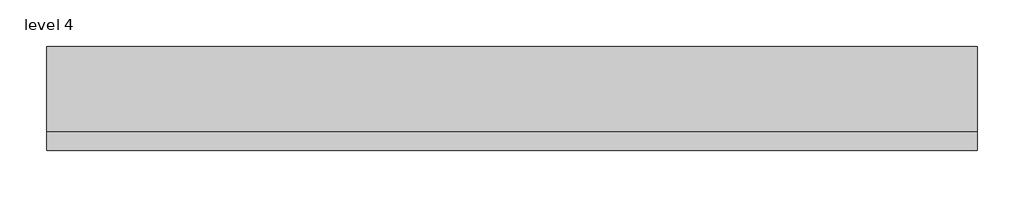
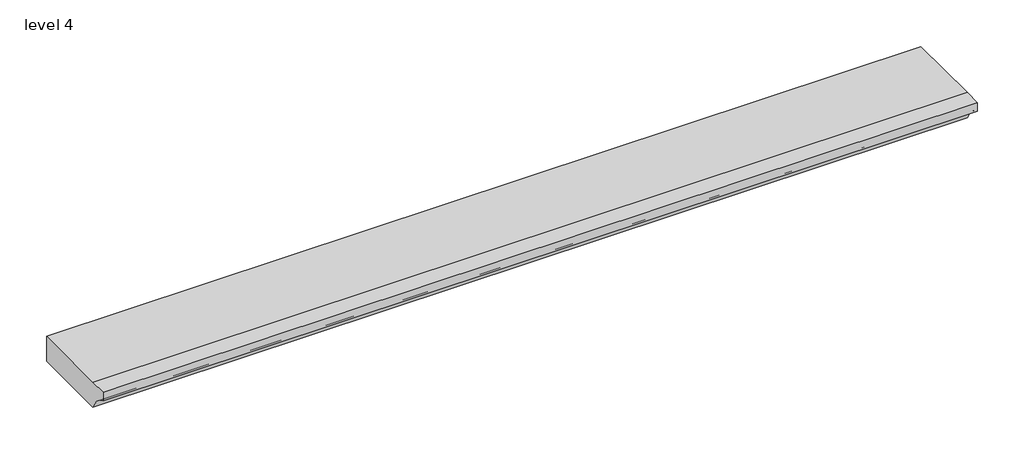
# One storey: 1 proxy.
"""IFC4 building model written with IfcOpenShell, lengths in millimetres."""

from ifc_helpers import new_model, si_unit, origin, place, context, project, spatial, transform, mapped, element, save
from components import generic_models_5_generic_models_5_b956d3bb

model = new_model("IFC4")

# Units and contexts
model_context = context("Model", 3, world=origin())
ifc_project = project(units=[si_unit("LENGTHUNIT", "METRE", prefix="MILLI")], contexts=[model_context])

# Site, building, storey
site = spatial("IfcSite", under=ifc_project)
building = spatial("IfcBuilding", under=site)
storey = spatial("IfcBuildingStorey", under=building, Name="level 4", Elevation=7467.6)

# Proxy
placement = place(None, origin())
generic_models_5_generic_models_5_shape = generic_models_5_generic_models_5_b956d3bb(model_context)
element("IfcBuildingElementProxy", 1, Name="Generic Models 5 : Generic Models 5", ObjectType="Generic Models 5 : Generic Models 5", at=placement, inside=storey, context=model_context, shape_type="MappedRepresentation", body=[
    mapped(generic_models_5_generic_models_5_shape, transform((0.0, 0.0, 0.0), x_axis=(1.0, 0.0, 0.0), y_axis=(0.0, 1.0, 0.0), z_axis=(0.0, 0.0, 1.0))),
])

save(model, "model.ifc")

# Revit data of these elements
# Element 1 (IfcBuildingElementProxy, "Generic Models 5 : Generic Models 5")
#   Phase Created = New Construction
